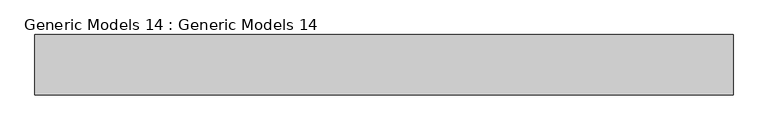
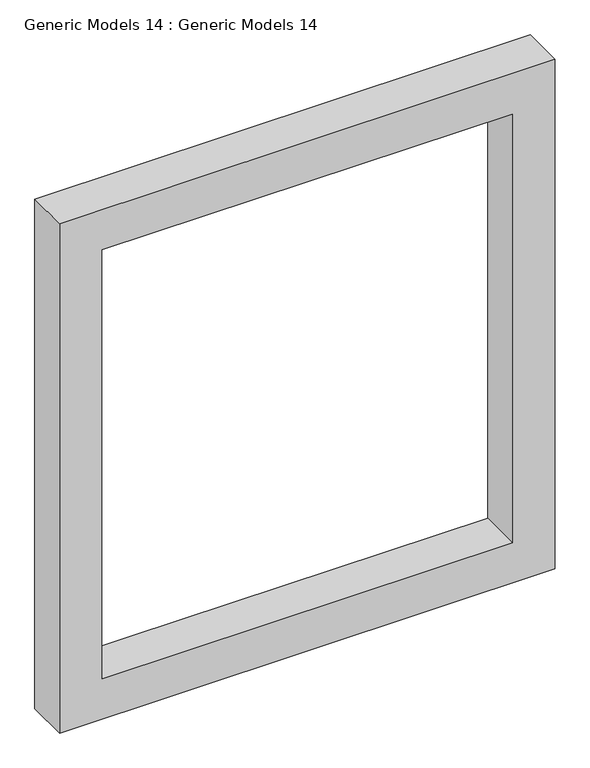
"""IFC4 building model written with IfcOpenShell, lengths in millimetres: proxy geometry, Generic Models 14 : Generic Models 14."""

from ifc_helpers import new_model, si_unit, frame, origin, place, context, project, spatial, polyline, outline, extrude, source, transform, mapped, element, save


def generic_models_14_generic_models_14_97bd1c4e(model_context):
    return source(origin(), model_context, "Body", "SweptSolid", [
        extrude(outline(polyline([(5740.4, -4872.1482439), (4140.2, -4872.1482439), (4140.2, -3398.9482439), (5740.4, -3398.9482439), (5740.4, -4872.1482439)]), holes=[polyline([(5613.4, -4745.1482439), (5613.4, -3525.9482439), (4267.2, -3525.9482439), (4267.2, -4745.1482439), (5613.4, -4745.1482439)])]), frame((0.0, 7791.8047538, 0.0), z_axis=(0.0, 1.0, 0.0), x_axis=(0.0, 0.0, 1.0)), (0.0, 0.0, 1.0), 127.0),
    ])


if __name__ == "__main__":
    model = new_model("IFC4")
    model_context = context("Model", 3, world=origin())
    ifc_project = project(units=[si_unit("LENGTHUNIT", "METRE", prefix="MILLI")], contexts=[model_context])
    site = spatial("IfcSite", under=ifc_project)
    building = spatial("IfcBuilding", under=site)
    placement = place(None, origin())
    generic_models_14_generic_models_14_shape = generic_models_14_generic_models_14_97bd1c4e(model_context)
    element("IfcBuildingElementProxy", 1, Name="Generic Models 14 : Generic Models 14", ObjectType="Generic Models 14 : Generic Models 14", at=placement, inside=building, context=model_context, shape_type="MappedRepresentation", body=[
        mapped(generic_models_14_generic_models_14_shape, transform((0.0, 0.0, 0.0), x_axis=(1.0, 0.0, 0.0), y_axis=(0.0, 1.0, 0.0), z_axis=(0.0, 0.0, 1.0))),
    ])
    save(model, "model.ifc")

# Revit data of these elements
# Element 1 (IfcBuildingElementProxy, "Generic Models 14 : Generic Models 14")
#   Materials on its faces: "BLACK"
# Materials
#   "BLACK": class "Generic", colour RGB 120 120 120, transparency 0, Cost = 0
